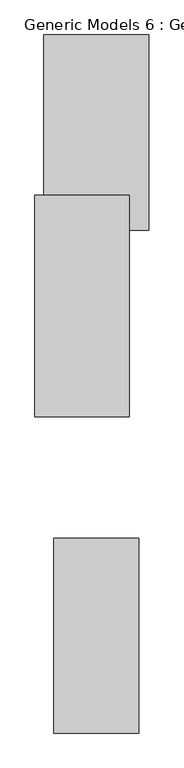
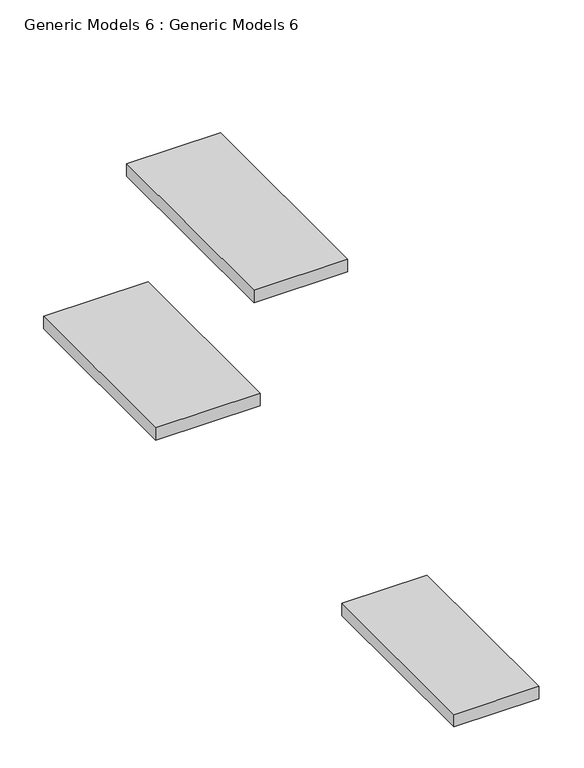
"""IFC4 building model written with IfcOpenShell, lengths in millimetres: proxy geometry, Generic Models 6 : Generic Models 6."""

from ifc_helpers import new_model, si_unit, frame, origin, place, context, project, spatial, polyline, outline, extrude, source, transform, mapped, element, save


def generic_models_6_generic_models_6_d9953a67(model_context):
    return source(origin(), model_context, "Body", "SweptSolid", [
        extrude(outline(polyline([(-24341.8386697, -8786.8858751), (-23351.2386697, -8786.8858751), (-23351.2386697, -11048.9511954), (-24341.8386697, -11048.9511954), (-24341.8386697, -8786.8858751)])), frame((0.0, 0.0, 2393.4159661), z_axis=(0.0, 0.0, 1.0), x_axis=(1.0, 0.0, 0.0)), (0.0, 0.0, 1.0), 152.4),
        extrude(outline(polyline([(-24456.1386697, -2948.7393216), (-23236.9386697, -2948.7393216), (-23236.9386697, -5213.3011954), (-24456.1386697, -5213.3011954), (-24456.1386697, -2948.7393216)])), frame((0.0, 0.0, 2430.0392006), z_axis=(0.0, 0.0, 1.0), x_axis=(1.0, 0.0, 0.0)), (0.0, 0.0, 1.0), 152.4),
        extrude(outline(polyline([(-24557.7386697, -4807.7322685), (-23465.5386697, -4807.7322685), (-23465.5386697, -7378.6511954), (-24557.7386697, -7378.6511954), (-24557.7386697, -4807.7322685)])), frame((0.0, 0.0, 5474.6486322), z_axis=(0.0, 0.0, 1.0), x_axis=(1.0, 0.0, 0.0)), (0.0, 0.0, 1.0), 152.4),
    ])


if __name__ == "__main__":
    model = new_model("IFC4")
    model_context = context("Model", 3, world=origin())
    ifc_project = project(units=[si_unit("LENGTHUNIT", "METRE", prefix="MILLI")], contexts=[model_context])
    site = spatial("IfcSite", under=ifc_project)
    building = spatial("IfcBuilding", under=site)
    placement = place(None, origin())
    generic_models_6_generic_models_6_shape = generic_models_6_generic_models_6_d9953a67(model_context)
    element("IfcBuildingElementProxy", 1, Name="Generic Models 6 : Generic Models 6", ObjectType="Generic Models 6 : Generic Models 6", at=placement, inside=building, context=model_context, shape_type="MappedRepresentation", body=[
        mapped(generic_models_6_generic_models_6_shape, transform((0.0, 0.0, 0.0), x_axis=(1.0, 0.0, 0.0), y_axis=(0.0, 1.0, 0.0), z_axis=(0.0, 0.0, 1.0))),
    ])
    save(model, "model.ifc")
